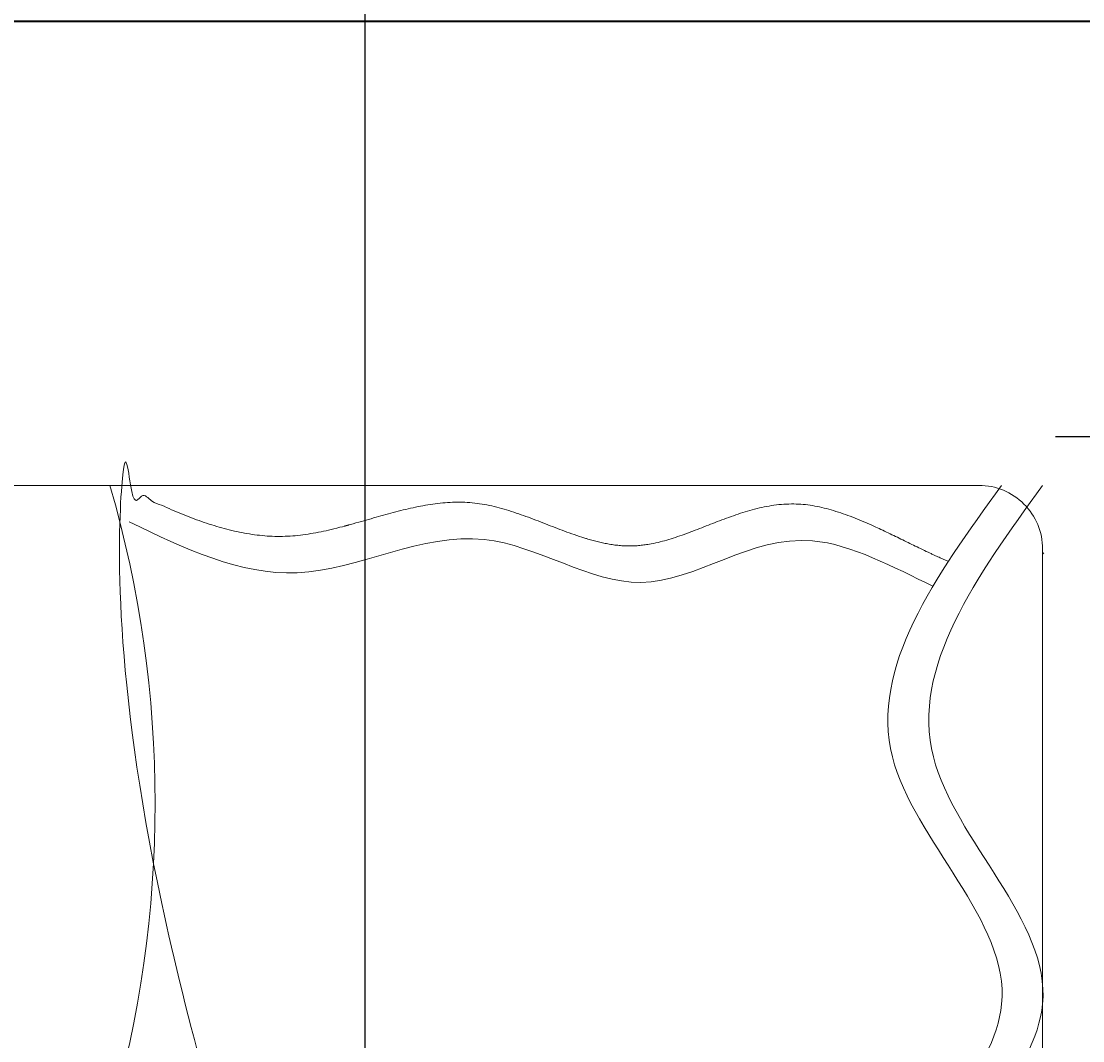
# Model space of a CAD drawing. Units: inches. Extents: x -61 to 1599, y -1316 to 257.
# Tile 151 of 204: x 440 to 490, y 101 to 149. Entities that reach past the tile are written whole.
import ezdxf

# ---------------------------------------------------------------- set-up
doc = ezdxf.new("R2010")
doc.units = ezdxf.units.IN
doc.header["$MEASUREMENT"] = 0
for name, color, linetype, lineweight in [('A-ANNO-DIMS', 2, 'Continuous', 18), ('FURNITURE', 83, 'Continuous', 18), ('WALLS', 4, 'Continuous', 35)]:
    doc.layers.add(name, color=color, linetype=linetype, lineweight=lineweight)
doc.styles.get("Standard").update_dxf_attribs({"font": 'arial.ttf'})
doc.dimstyles.get("Standard").update_dxf_attribs({"dimtxt": 0.18, "dimasz": 0.18, "dimexe": 0.18, "dimexo": 0.0625, "dimgap": 0.09, "dimtad": 0, "dimtih": 1, "dimtoh": 1, "dimdec": 0, "dimzin": 0, "dimdsep": 46, "dimlunit": 3, "dimtxsty": 'Standard', "dimcen": 0.09, "dimadec": 0, "dimazin": 0, "dimtfac": 1, "dimtdec": 0, "dimtofl": 0, "dimtmove": 0, "dimatfit": 3, "dimfxl": 1, "dimtolj": 1, "dimtzin": 0, "dimarcsym": 0})

# ---------------------------------------------------------------- blocks, each defined once
blk = doc.blocks.new('BED-DOUBLE-COMPACT')
blk.add_lwpolyline([(77, 60.036), (3, 60.036, 0.414214), (0, 57.036), (0, 3.036, 0.414214), (3, 0.036), (77, 0.036, 0.414214), (80, 3.036), (80, 57.036, 0.414214)], format="xyb", close=True)
blk.add_lwpolyline([(35.995, 0.036, -0.22309), (35.995, 30.036, 0.142156), (35.995, 60.036)], format="xyb")
blk.add_rational_spline([(50.356, 0.036), (44.305, 9.081), (39.572, 18.88), (36.247, 29.242), (36.329, 29.431), (36.413, 29.619), (36.498, 29.807), (39.384, 39.751), (39.361, 50.105), (36.431, 60.036), (39.05, 58.775), (44.504, 56.147), (52.793, 61.024), (60.854, 55.204), (67.651, 61.048), (73.388, 57.356), (75.556, 56.449)], [1, 0.993520320424, 0.993520320424, 1, 0.99997444972, 0.99997444972, 1, 0.973174868659, 0.973174868659, 1, 1, 1, 1, 1, 1, 1, 1], degree=3, knots=[0, 0, 0, 0, 0.279074, 0.279074, 0.279074, 0.296584, 0.296584, 0.296584, 0.865868, 0.865868, 0.865868, 9.142578, 18.107734, 25.769226, 34.110801, 40.441511, 40.441511, 40.441511, 40.441511])
for points, knots in [([(78.068, 0.036), (75.8, 2.259), (70.917, 7.043), (82.188, 15.495), (70.028, 25.556), (82.2, 36.262), (68.972, 47.493), (74.957, 55.746), (78.068, 60.036)], [0, 0, 0, 0, 7.980285, 17.179806, 28.830278, 39.318084, 52.078264, 65.891546, 65.891546, 65.891546, 65.891546]), ([(80, 0.036), (77.732, 2.259), (72.849, 7.043), (84.121, 15.495), (71.96, 25.556), (84.132, 36.262), (70.904, 47.493), (76.889, 55.746), (80, 60.036)], [0, 0, 0, 0, 7.980285, 17.179806, 28.830278, 39.318084, 52.078264, 65.891546, 65.891546, 65.891546, 65.891546]), ([(36.908, 58.315), (39.526, 57.053), (44.981, 54.425), (53.27, 59.302), (61.331, 53.483), (67.779, 59.026), (72.974, 56.167), (74.826, 55.276)], [0, 0, 0, 0, 8.27671, 17.241866, 24.903358, 33.244933, 38.427294, 38.427294, 38.427294, 38.427294])]:
    blk.add_open_spline(points, degree=3, knots=knots)
blk.add_open_spline([(80, 56.785), (80.017, 56.806), (80.034, 56.828), (80.051, 56.85)], degree=3)
blk = doc.blocks.new('*D677')
at = {"layer": 'A-ANNO-DIMS', "color": 0, "lineweight": -2, "transparency": 16777216}
for p, q in [((488.407, 129.084), (500.607, 129.084)), ((500.427, 128.904), (500.427, 98.089)), ((500.427, 66.909), (500.427, 97.725)), ((488.407, 66.729), (500.607, 66.729))]:
    blk.add_line(p, q, dxfattribs=at)
at = {"layer": 'A-ANNO-DIMS', "color": 0, "transparency": 16777216}
for points in [[(500.397, 128.904), (500.457, 128.904), (500.427, 129.084)], [(500.397, 66.909), (500.457, 66.909), (500.427, 66.729)]]:
    blk.add_solid(points, dxfattribs=at)
at = {"layer": 'DEFPOINTS', "color": 0, "transparency": 16777216}
for p in [(488.345, 129.084), (500.427, 129.084), (488.345, 66.729)]:
    blk.add_point(p, dxfattribs=at)
at = {"layer": 'A-ANNO-DIMS', "color": 0, "transparency": 16777216, "insert": (500.427, 97.907), "char_height": 0.18, "attachment_point": 5}
blk.add_mtext('\\A1;62 TYP.', dxfattribs=at)
blk = doc.blocks.new('*D703')
at = {"layer": 'A-ANNO-DIMS', "color": 0, "lineweight": -2, "transparency": 16777216}
for p, q in [((372.32, -616.882), (372.32, 257.457)), ((455.833, -616.882), (455.833, 257.457)), ((372.5, 257.277), (413.7, 257.277)), ((455.653, 257.277), (414.453, 257.277))]:
    blk.add_line(p, q, dxfattribs=at)
at = {"layer": 'A-ANNO-DIMS', "color": 0, "transparency": 16777216}
for points in [[(372.5, 257.307), (372.5, 257.247), (372.32, 257.277)], [(455.653, 257.307), (455.653, 257.247), (455.833, 257.277)]]:
    blk.add_solid(points, dxfattribs=at)
at = {"layer": 'DEFPOINTS', "color": 0, "transparency": 16777216}
for p in [(455.833, 257.277), (372.32, -616.945), (455.833, -616.945)]:
    blk.add_point(p, dxfattribs=at)
at = {"layer": 'A-ANNO-DIMS', "color": 0, "transparency": 16777216, "insert": (414.076, 257.277), "char_height": 0.18, "attachment_point": 5}
blk.add_mtext('\\A1;83.51', dxfattribs=at)

msp = doc.modelspace()

# ---------------------------------------------------------------- linework, layer by layer
at = {"layer": 'WALLS'}
msp.add_line((403.7028, 148.6771), (535.7028, 148.6771), dxfattribs=at)

# ---------------------------------------------------------------- block references
at = {"layer": 'FURNITURE'}
msp.add_blockref('BED-DOUBLE-COMPACT', (407.794, 66.733), dxfattribs=at)

# ---------------------------------------------------------------- dimensions: what is measured, and where the dimension line sits
at = {"layer": 'A-ANNO-DIMS'}
dim = msp.add_linear_dim(base=(455.8327, 257.2771), p1=(372.3201, -616.9446), p2=(455.8327, -616.9446), dimstyle='Standard', override={"dimdec": 2, "dimlfac": 1, "dimrnd": 0, "dimzin": 0, "dimdsep": 46, "dimlunit": 2}, dxfattribs=at)
dim.commit()
dim.dimension.update_dxf_attribs({"geometry": '*D703', "text_midpoint": (414.0764, 257.2771)})
dim = msp.add_linear_dim(base=(500.4274, 129.084), p1=(488.3448, 66.7295), p2=(488.3448, 129.084), angle=90, text='<> TYP.', dimstyle='Standard', override={"dimdec": 0, "dimlfac": 1, "dimrnd": 0, "dimzin": 0, "dimdsep": 46, "dimlunit": 2}, dxfattribs=at)
dim.commit()
dim.dimension.update_dxf_attribs({"geometry": '*D677', "text_midpoint": (500.4274, 97.9068)})

doc.saveas('drawing.dxf')
